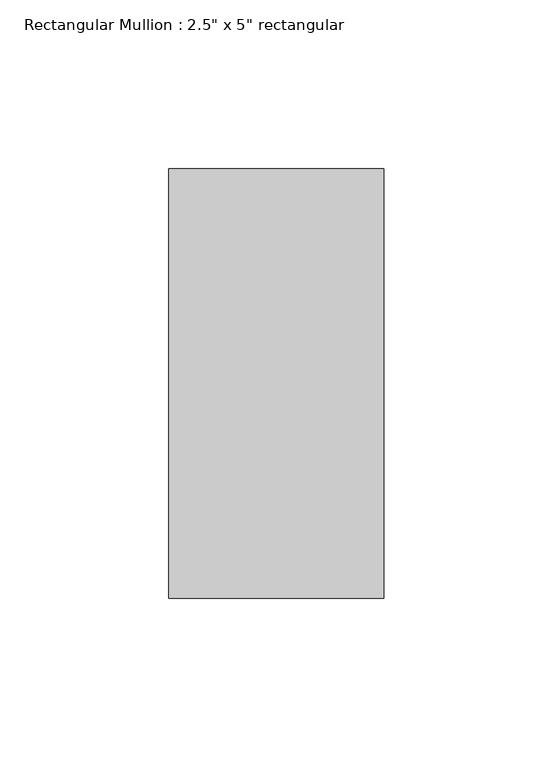
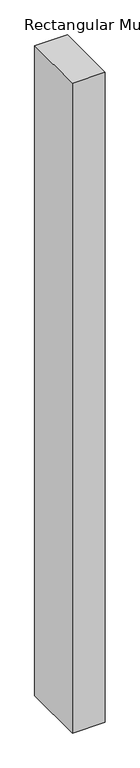
"""IFC4 building model written with IfcOpenShell, lengths in millimetres: member geometry."""

from ifc_helpers import new_model, si_unit, frame, origin, place, context, project, spatial, polyline, outline, extrude, source, transform, mapped, element, save


def member_c919ac1a(model_context):
    return source(origin(), model_context, "Body", "SweptSolid", [
        extrude(outline(polyline([(0.0, 63.5), (0.0, -63.5), (-63.5, -63.5), (-63.5, 63.5), (0.0, 63.5)])), frame((0.0, 0.0, -1334.5583333), z_axis=(0.0, 0.0, 1.0), x_axis=(1.0, 0.0, 0.0)), (0.0, 0.0, 1.0), 1334.5583333),
    ])


if __name__ == "__main__":
    model = new_model("IFC4")
    model_context = context("Model", 3, world=origin())
    ifc_project = project(units=[si_unit("LENGTHUNIT", "METRE", prefix="MILLI")], contexts=[model_context])
    site = spatial("IfcSite", under=ifc_project)
    building = spatial("IfcBuilding", under=site)
    placement = place(None, origin())
    member_shape = member_c919ac1a(model_context)
    element("IfcMember", 1, ObjectType="Rectangular Mullion : 2.5\" x 5\" rectangular", at=placement, inside=building, context=model_context, shape_type="MappedRepresentation", body=[
        mapped(member_shape, transform((0.0, 0.0, 0.0), x_axis=(1.0, 0.0, 0.0), y_axis=(0.0, 1.0, 0.0), z_axis=(0.0, 0.0, 1.0))),
    ])
    save(model, "model.ifc")

# Revit data of these elements
# Type "Rectangular Mullion : 2.5\" x 5\" rectangular"
#   built-in parameter 1007304 = 0.416667 (stored number, unit not read)
#   built-in parameter 1007301 = 0.104167 (stored number, unit not read)
#   built-in parameter 1007300 = 0.104167 (stored number, unit not read)
# Element 1 (IfcMember, "Rectangular Mullion : 2.5\" x 5\" rectangular")
#   Materials on its faces: "BLACK MATERIAL"
# Materials
#   "BLACK MATERIAL": class "Generic", colour RGB 120 120 120, transparency 0, Cost = 0
